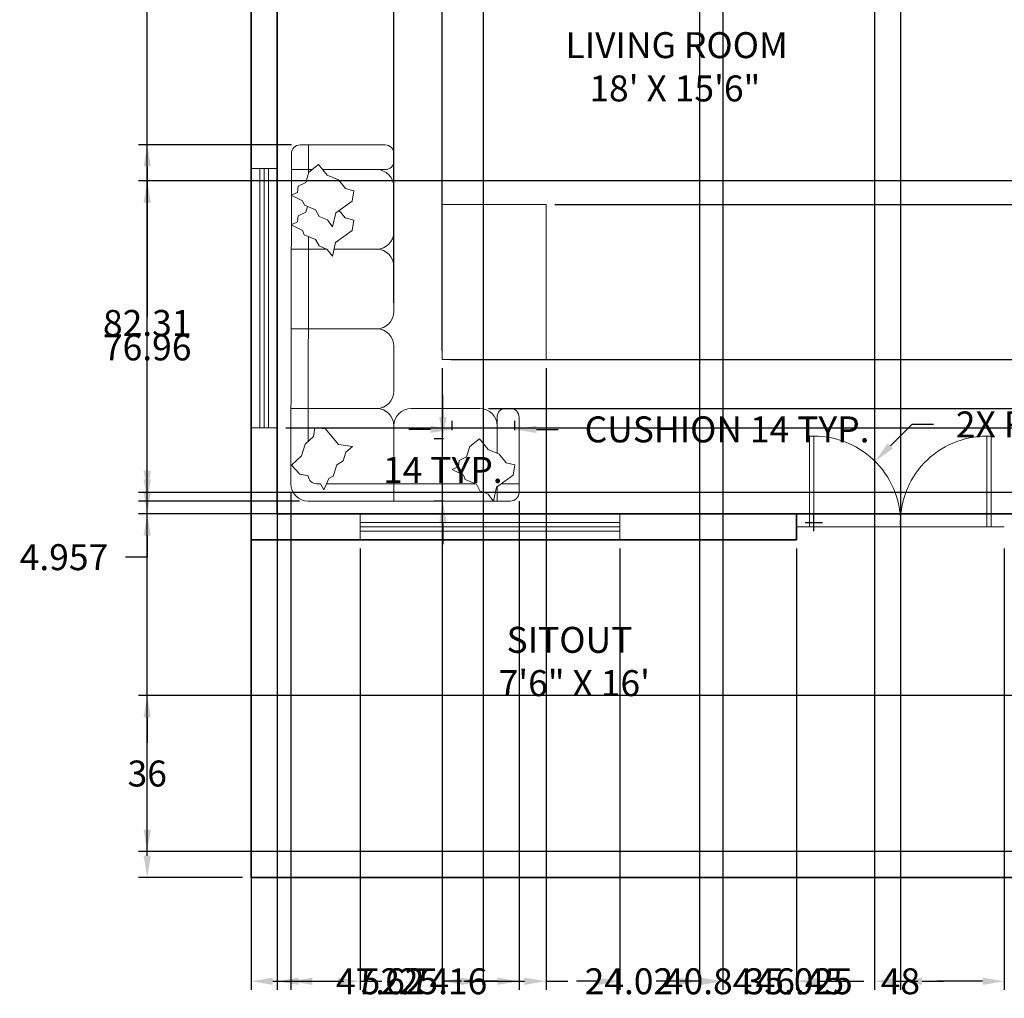
# Model space of a CAD drawing. Units: inches. Extents: x 185 to 668, y 153 to 689.
# Tile 1 of 5: x 190 to 417, y 153 to 380. Entities that reach past the tile are written whole.
import ezdxf

# ---------------------------------------------------------------- set-up
doc = ezdxf.new("R2010")
doc.units = ezdxf.units.IN
doc.header["$MEASUREMENT"] = 0
for name, color, linetype, lineweight in [('A-ANNO-DIMS', 2, 'Continuous', 18), ('A-AREA-IDEN', 7, 'Continuous', 25), ('A-DOOR', 3, 'Continuous', 18), ('A-FURN', 8, 'Continuous', 18), ('A-GLAZ', 4, 'Continuous', 18), ('A-WALL', 7, 'Continuous', 35)]:
    doc.layers.add(name, color=color, linetype=linetype, lineweight=lineweight)
doc.styles.get("Standard").update_dxf_attribs({"font": 'arial.ttf'})
doc.dimstyles.get("Standard").update_dxf_attribs({"dimtxt": 6, "dimasz": 5, "dimexe": 2, "dimexo": 2, "dimgap": 4, "dimtad": 0, "dimtih": 1, "dimtoh": 1, "dimdec": 0, "dimzin": 0, "dimdsep": 46, "dimlunit": 3, "dimtxsty": 'Standard', "dimcen": 2, "dimadec": 0, "dimazin": 0, "dimtfac": 1, "dimtdec": 0, "dimtofl": 0, "dimtmove": 0, "dimatfit": 3, "dimfxl": 1, "dimtolj": 1, "dimtzin": 0, "dimarcsym": 0})

# ---------------------------------------------------------------- blocks, each defined once
blk = doc.blocks.new('CUSHION-SOFA')
for p, q in [((6.28, 14.39), (4.07, 12.61)), ((6.28, 14.39), (8.27, 11.92)), ((4.07, 12.61), (3.33, 10.2)), ((8.27, 11.92), (10.87, 10.84)), ((1.59, 9.37), (1.41, 7.95)), ((3.33, 10.2), (1.59, 9.37)), ((10.87, 10.84), (12.49, 8.85)), ((1.41, 7.95), (0, 7.29)), ((0, 7.29), (2.58, 5.99)), ((12.49, 8.85), (14.45, 8.34)), ((14.09, 5.96), (14.45, 8.34)), ((2.58, 5.99), (3.01, 4.98)), ((3.01, 4.98), (5.57, 3.91)), ((10.25, 3.2), (14.09, 5.96)), ((5.57, 3.91), (6.41, 2.39)), ((6.41, 2.39), (8.33, 1.6)), ((9.53, 0), (10.25, 3.2)), ((8.33, 1.6), (9.53, 0))]:
    blk.add_line(p, q)
blk = doc.blocks.new('WINDOW-60')
for p, q in [((2, 60), (0, 60)), ((2, 60), (2, 0)), ((4, 60), (2, 60)), ((3, 0), (3, 60)), ((4, 0), (4, 60)), ((4, 60), (6, 60)), ((6, 0), (0, 0)), ((2, 0), (0, 0)), ((2, 0), (4, 0)), ((4, 0), (6, 0))]:
    blk.add_line(p, q)
blk = doc.blocks.new('*D17')
at = {"layer": 'A-ANNO-DIMS', "color": 0, "lineweight": -2, "transparency": 16777216}
for p, q in [((289.49, 284.74), (289.49, 286.91)), ((303.94, 284.74), (303.94, 286.91)), ((284.49, 284.91), (279.49, 284.91)), ((308.94, 284.91), (313.94, 284.91))]:
    blk.add_line(p, q, dxfattribs=at)
at = {"layer": 'A-ANNO-DIMS', "color": 0, "transparency": 16777216}
for points in [[(284.49, 285.74), (284.49, 284.08), (289.49, 284.91)], [(308.94, 285.74), (308.94, 284.08), (303.94, 284.91)]]:
    blk.add_solid(points, dxfattribs=at)
at = {"layer": 'Defpoints', "color": 0, "transparency": 16777216}
for p in [(303.94, 284.91), (289.49, 282.74), (303.94, 282.74)]:
    blk.add_point(p, dxfattribs=at)
at = {"layer": 'A-ANNO-DIMS', "color": 0, "transparency": 16777216, "insert": (352.99, 284.91), "char_height": 6, "attachment_point": 5}
blk.add_mtext('\\A1;CUSHION 14 TYP.', dxfattribs=at)
blk = doc.blocks.new('*D18')
at = {"layer": 'A-ANNO-DIMS', "color": 0, "lineweight": -2, "transparency": 16777216}
for p, q in [((287.32, 287.74), (287.32, 292.74)), ((287.49, 282.74), (285.32, 282.74)), ((287.49, 268.35), (285.32, 268.35)), ((287.32, 263.35), (287.32, 258.35))]:
    blk.add_line(p, q, dxfattribs=at)
at = {"layer": 'A-ANNO-DIMS', "color": 0, "transparency": 16777216}
for points in [[(286.49, 287.74), (288.16, 287.74), (287.32, 282.74)], [(286.49, 263.35), (288.16, 263.35), (287.32, 268.35)]]:
    blk.add_solid(points, dxfattribs=at)
at = {"layer": 'Defpoints', "color": 0, "transparency": 16777216}
for p in [(287.32, 282.74), (289.49, 282.74), (289.49, 268.35)]:
    blk.add_point(p, dxfattribs=at)
at = {"layer": 'A-ANNO-DIMS', "color": 0, "transparency": 16777216, "insert": (287.32, 275.55), "char_height": 6, "attachment_point": 5}
blk.add_mtext('\\A1;14 TYP.', dxfattribs=at)
blk = doc.blocks.new('*D26')
at = {"layer": 'A-ANNO-DIMS', "color": 0, "lineweight": -2, "transparency": 16777216}
for p, q in [((241.04, 661.38), (217.02, 661.38)), ((219.02, 656.38), (219.02, 428.44)), ((219.02, 186.38), (219.02, 414.32)), ((241.04, 181.38), (217.02, 181.38))]:
    blk.add_line(p, q, dxfattribs=at)
at = {"layer": 'A-ANNO-DIMS', "color": 0, "transparency": 16777216}
for points in [[(218.19, 656.38), (219.86, 656.38), (219.02, 661.38)], [(218.19, 186.38), (219.86, 186.38), (219.02, 181.38)]]:
    blk.add_solid(points, dxfattribs=at)
at = {"layer": 'Defpoints', "color": 0, "transparency": 16777216}
for p in [(219.02, 661.38), (243.04, 661.38), (243.04, 181.38)]:
    blk.add_point(p, dxfattribs=at)
at = {"layer": 'A-ANNO-DIMS', "color": 0, "transparency": 16777216, "insert": (219.02, 421.38), "char_height": 6, "attachment_point": 5}
blk.add_mtext('\\A1;480', dxfattribs=at)
blk = doc.blocks.new('*D28')
at = {"layer": 'A-ANNO-DIMS', "color": 0, "lineweight": -2, "transparency": 16777216}
for p, q in [((627.06, 285.24), (627.06, 290.24)), ((627.06, 290.24), (632.06, 290.24)), ((251.04, 285.24), (629.06, 285.24)), ((627.06, 270.38), (627.06, 280.24)), ((251.04, 265.38), (629.06, 265.38))]:
    blk.add_line(p, q, dxfattribs=at)
at = {"layer": 'A-ANNO-DIMS', "color": 0, "transparency": 16777216}
for points in [[(626.23, 280.24), (627.89, 280.24), (627.06, 285.24)], [(626.23, 270.38), (627.89, 270.38), (627.06, 265.38)]]:
    blk.add_solid(points, dxfattribs=at)
at = {"layer": 'Defpoints', "color": 0, "transparency": 16777216}
for p in [(249.04, 285.24), (627.06, 285.24), (249.04, 265.38)]:
    blk.add_point(p, dxfattribs=at)
at = {"layer": 'A-ANNO-DIMS', "color": 0, "transparency": 16777216, "insert": (645.9, 290.24), "char_height": 6, "attachment_point": 5}
blk.add_mtext('\\A1;19.86', dxfattribs=at)
blk = doc.blocks.new('*D32')
at = {"layer": 'A-ANNO-DIMS', "color": 0, "lineweight": -2, "transparency": 16777216}
for p, q in [((352.02, 653.38), (352.02, 155.36)), ((387.04, 653.38), (387.04, 155.36)), ((347.02, 157.36), (342.02, 157.36)), ((392.04, 157.36), (397.04, 157.36))]:
    blk.add_line(p, q, dxfattribs=at)
at = {"layer": 'A-ANNO-DIMS', "color": 0, "transparency": 16777216}
for points in [[(347.02, 158.19), (347.02, 156.53), (352.02, 157.36)], [(392.04, 158.19), (392.04, 156.53), (387.04, 157.36)]]:
    blk.add_solid(points, dxfattribs=at)
at = {"layer": 'Defpoints', "color": 0, "transparency": 16777216}
for p in [(352.02, 655.38), (387.04, 655.38), (387.04, 157.36)]:
    blk.add_point(p, dxfattribs=at)
at = {"layer": 'A-ANNO-DIMS', "color": 0, "transparency": 16777216, "insert": (369.53, 157.36), "char_height": 6, "attachment_point": 5}
blk.add_mtext('\\A1;35.025', dxfattribs=at)
blk = doc.blocks.new('*D34')
at = {"layer": 'A-ANNO-DIMS', "color": 0, "lineweight": -2, "transparency": 16777216}
for p, q in [((243.04, 257.38), (243.04, 155.36)), ((268.2, 257.38), (268.2, 155.36)), ((248.04, 157.36), (263.2, 157.36)), ((268.2, 157.36), (273.2, 157.36))]:
    blk.add_line(p, q, dxfattribs=at)
at = {"layer": 'A-ANNO-DIMS', "color": 0, "transparency": 16777216}
for points in [[(248.04, 158.19), (248.04, 156.53), (243.04, 157.36)], [(263.2, 158.19), (263.2, 156.53), (268.2, 157.36)]]:
    blk.add_solid(points, dxfattribs=at)
at = {"layer": 'Defpoints', "color": 0, "transparency": 16777216}
for p in [(243.04, 259.38), (268.2, 259.38), (268.2, 157.36)]:
    blk.add_point(p, dxfattribs=at)
at = {"layer": 'A-ANNO-DIMS', "color": 0, "transparency": 16777216, "insert": (287.37, 157.36), "char_height": 6, "attachment_point": 5}
blk.add_mtext('\\A1;25.16', dxfattribs=at)
blk = doc.blocks.new('*D35')
at = {"layer": 'A-ANNO-DIMS', "color": 0, "lineweight": -2, "transparency": 16777216}
for p, q in [((328.2, 257.38), (328.2, 155.36)), ((369.04, 257.38), (369.04, 155.36)), ((323.2, 157.36), (318.2, 157.36)), ((374.04, 157.36), (379.04, 157.36))]:
    blk.add_line(p, q, dxfattribs=at)
at = {"layer": 'A-ANNO-DIMS', "color": 0, "transparency": 16777216}
for points in [[(323.2, 158.19), (323.2, 156.53), (328.2, 157.36)], [(374.04, 158.19), (374.04, 156.53), (369.04, 157.36)]]:
    blk.add_solid(points, dxfattribs=at)
at = {"layer": 'Defpoints', "color": 0, "transparency": 16777216}
for p in [(328.2, 259.38), (369.04, 259.38), (369.04, 157.36)]:
    blk.add_point(p, dxfattribs=at)
at = {"layer": 'A-ANNO-DIMS', "color": 0, "transparency": 16777216, "insert": (348.62, 157.36), "char_height": 6, "attachment_point": 5}
blk.add_mtext('\\A1;40.84', dxfattribs=at)
blk = doc.blocks.new('*D36')
at = {"layer": 'A-ANNO-DIMS', "color": 0, "lineweight": -2, "transparency": 16777216}
for p, q in [((369.04, 257.38), (369.04, 155.36)), ((417.04, 257.38), (417.04, 155.36)), ((374.04, 157.36), (384.62, 157.36)), ((412.04, 157.36), (401.47, 157.36))]:
    blk.add_line(p, q, dxfattribs=at)
at = {"layer": 'A-ANNO-DIMS', "color": 0, "transparency": 16777216}
for points in [[(374.04, 158.19), (374.04, 156.53), (369.04, 157.36)], [(412.04, 158.19), (412.04, 156.53), (417.04, 157.36)]]:
    blk.add_solid(points, dxfattribs=at)
at = {"layer": 'Defpoints', "color": 0, "transparency": 16777216}
for p in [(369.04, 259.38), (417.04, 259.38), (417.04, 157.36)]:
    blk.add_point(p, dxfattribs=at)
at = {"layer": 'A-ANNO-DIMS', "color": 0, "transparency": 16777216, "insert": (393.04, 157.36), "char_height": 6, "attachment_point": 5}
blk.add_mtext('\\A1;48', dxfattribs=at)
blk = doc.blocks.new('*D53')
at = {"layer": 'A-ANNO-DIMS', "color": 0, "lineweight": -2, "transparency": 16777216}
for p, q in [((457.04, 342.34), (217.02, 342.34)), ((219.02, 337.34), (219.02, 310.92)), ((219.02, 270.38), (219.02, 296.79)), ((457.04, 265.38), (217.02, 265.38))]:
    blk.add_line(p, q, dxfattribs=at)
at = {"layer": 'A-ANNO-DIMS', "color": 0, "transparency": 16777216}
for points in [[(218.19, 337.34), (219.86, 337.34), (219.02, 342.34)], [(218.19, 270.38), (219.86, 270.38), (219.02, 265.38)]]:
    blk.add_solid(points, dxfattribs=at)
at = {"layer": 'Defpoints', "color": 0, "transparency": 16777216}
for p in [(219.02, 342.34), (459.04, 342.34), (459.04, 265.38)]:
    blk.add_point(p, dxfattribs=at)
at = {"layer": 'A-ANNO-DIMS', "color": 0, "transparency": 16777216, "insert": (219.02, 303.86), "char_height": 6, "attachment_point": 5}
blk.add_mtext('\\A1;76.96', dxfattribs=at)
blk = doc.blocks.new('*D54')
at = {"layer": 'A-ANNO-DIMS', "color": 0, "lineweight": -2, "transparency": 16777216}
for p, q in [((287.14, 299.05), (287.14, 155.36)), ((311.16, 299.05), (311.16, 155.36)), ((292.14, 157.36), (306.16, 157.36)), ((311.16, 157.36), (316.16, 157.36))]:
    blk.add_line(p, q, dxfattribs=at)
at = {"layer": 'A-ANNO-DIMS', "color": 0, "transparency": 16777216}
for points in [[(292.14, 158.19), (292.14, 156.53), (287.14, 157.36)], [(306.16, 158.19), (306.16, 156.53), (311.16, 157.36)]]:
    blk.add_solid(points, dxfattribs=at)
at = {"layer": 'Defpoints', "color": 0, "transparency": 16777216}
for p in [(287.14, 301.05), (311.16, 301.05), (311.16, 157.36)]:
    blk.add_point(p, dxfattribs=at)
at = {"layer": 'A-ANNO-DIMS', "color": 0, "transparency": 16777216, "insert": (330.3, 157.36), "char_height": 6, "attachment_point": 5}
blk.add_mtext('\\A1;24.02', dxfattribs=at)
blk = doc.blocks.new('*D55')
at = {"layer": 'A-ANNO-DIMS', "color": 0, "lineweight": -2, "transparency": 16777216}
for p, q in [((313.16, 336.85), (629.06, 336.85)), ((627.06, 331.85), (627.06, 326.02)), ((627.06, 306.05), (627.06, 311.89)), ((313.16, 301.05), (629.06, 301.05))]:
    blk.add_line(p, q, dxfattribs=at)
at = {"layer": 'A-ANNO-DIMS', "color": 0, "transparency": 16777216}
for points in [[(626.23, 331.85), (627.89, 331.85), (627.06, 336.85)], [(626.23, 306.05), (627.89, 306.05), (627.06, 301.05)]]:
    blk.add_solid(points, dxfattribs=at)
at = {"layer": 'Defpoints', "color": 0, "transparency": 16777216}
for p in [(311.16, 336.85), (627.06, 336.85), (311.16, 301.05)]:
    blk.add_point(p, dxfattribs=at)
at = {"layer": 'A-ANNO-DIMS', "color": 0, "transparency": 16777216, "insert": (627.06, 318.95), "char_height": 6, "attachment_point": 5}
blk.add_mtext('\\A1;35.8', dxfattribs=at)
blk = doc.blocks.new('*D56')
at = {"layer": 'A-ANNO-DIMS', "color": 0, "lineweight": -2, "transparency": 16777216}
for p, q in [((252.19, 270.35), (252.19, 155.36)), ((304.93, 268.35), (304.93, 155.36)), ((257.19, 157.36), (264.45, 157.36)), ((299.93, 157.36), (292.67, 157.36))]:
    blk.add_line(p, q, dxfattribs=at)
at = {"layer": 'A-ANNO-DIMS', "color": 0, "transparency": 16777216}
for points in [[(257.19, 158.19), (257.19, 156.53), (252.19, 157.36)], [(299.93, 158.19), (299.93, 156.53), (304.93, 157.36)]]:
    blk.add_solid(points, dxfattribs=at)
at = {"layer": 'Defpoints', "color": 0, "transparency": 16777216}
for p in [(252.19, 272.35), (304.93, 270.35), (304.93, 157.36)]:
    blk.add_point(p, dxfattribs=at)
at = {"layer": 'A-ANNO-DIMS', "color": 0, "transparency": 16777216, "insert": (278.56, 157.36), "char_height": 6, "attachment_point": 5}
blk.add_mtext('\\A1;52.74', dxfattribs=at)
blk = doc.blocks.new('*D57')
at = {"layer": 'A-ANNO-DIMS', "color": 0, "lineweight": -2, "transparency": 16777216}
for p, q in [((252.32, 350.67), (217.02, 350.67)), ((219.02, 345.67), (219.02, 316.58)), ((219.02, 273.35), (219.02, 302.45)), ((254.19, 268.35), (217.02, 268.35))]:
    blk.add_line(p, q, dxfattribs=at)
at = {"layer": 'A-ANNO-DIMS', "color": 0, "transparency": 16777216}
for points in [[(218.19, 345.67), (219.86, 345.67), (219.02, 350.67)], [(218.19, 273.35), (219.86, 273.35), (219.02, 268.35)]]:
    blk.add_solid(points, dxfattribs=at)
at = {"layer": 'Defpoints', "color": 0, "transparency": 16777216}
for p in [(219.02, 350.67), (254.32, 350.67), (256.19, 268.35)]:
    blk.add_point(p, dxfattribs=at)
at = {"layer": 'A-ANNO-DIMS', "color": 0, "transparency": 16777216, "insert": (219.02, 309.51), "char_height": 6, "attachment_point": 5}
blk.add_mtext('\\A1;82.31', dxfattribs=at)
blk = doc.blocks.new('*D58')
at = {"layer": 'A-ANNO-DIMS', "color": 0, "lineweight": -2, "transparency": 16777216}
for p, q in [((276.02, 314.15), (276.02, 687.4)), ((287.14, 303.05), (287.14, 687.4)), ((271.02, 685.4), (266.02, 685.4)), ((292.14, 685.4), (297.14, 685.4))]:
    blk.add_line(p, q, dxfattribs=at)
at = {"layer": 'A-ANNO-DIMS', "color": 0, "transparency": 16777216}
for points in [[(271.02, 686.23), (271.02, 684.56), (276.02, 685.4)], [(292.14, 686.23), (292.14, 684.56), (287.14, 685.4)]]:
    blk.add_solid(points, dxfattribs=at)
at = {"layer": 'Defpoints', "color": 0, "transparency": 16777216}
for p in [(287.14, 685.4), (276.02, 312.15), (287.14, 301.05)]:
    blk.add_point(p, dxfattribs=at)
at = {"layer": 'A-ANNO-DIMS', "color": 0, "transparency": 16777216, "insert": (313.31, 685.4), "char_height": 6, "attachment_point": 5}
blk.add_mtext('\\A1;11.116', dxfattribs=at)
blk = doc.blocks.new('*D59')
at = {"layer": 'A-ANNO-DIMS', "color": 0, "lineweight": -2, "transparency": 16777216}
for p, q in [((627.06, 306.05), (627.06, 311.05)), ((289.14, 301.05), (629.06, 301.05)), ((297.85, 289.75), (629.06, 289.75)), ((627.06, 284.75), (627.06, 279.75)), ((627.06, 279.75), (622.06, 279.75))]:
    blk.add_line(p, q, dxfattribs=at)
at = {"layer": 'A-ANNO-DIMS', "color": 0, "transparency": 16777216}
for points in [[(626.23, 306.05), (627.89, 306.05), (627.06, 301.05)], [(626.23, 284.75), (627.89, 284.75), (627.06, 289.75)]]:
    blk.add_solid(points, dxfattribs=at)
at = {"layer": 'Defpoints', "color": 0, "transparency": 16777216}
for p in [(287.14, 301.05), (295.85, 289.75), (627.06, 289.75)]:
    blk.add_point(p, dxfattribs=at)
at = {"layer": 'A-ANNO-DIMS', "color": 0, "transparency": 16777216, "insert": (605.89, 279.75), "char_height": 6, "attachment_point": 5}
blk.add_mtext('\\A1;11.303', dxfattribs=at)
blk = doc.blocks.new('*D60')
at = {"layer": 'A-ANNO-DIMS', "color": 0, "lineweight": -2, "transparency": 16777216}
for p, q in [((439.04, 223.38), (217.02, 223.38)), ((219.02, 218.38), (219.02, 212.44)), ((219.02, 192.38), (219.02, 198.31)), ((439.04, 187.38), (217.02, 187.38))]:
    blk.add_line(p, q, dxfattribs=at)
at = {"layer": 'A-ANNO-DIMS', "color": 0, "transparency": 16777216}
for points in [[(218.19, 218.38), (219.86, 218.38), (219.02, 223.38)], [(218.19, 192.38), (219.86, 192.38), (219.02, 187.38)]]:
    blk.add_solid(points, dxfattribs=at)
at = {"layer": 'Defpoints', "color": 0, "transparency": 16777216}
for p in [(219.02, 223.38), (441.04, 223.38), (441.04, 187.38)]:
    blk.add_point(p, dxfattribs=at)
at = {"layer": 'A-ANNO-DIMS', "color": 0, "transparency": 16777216, "insert": (219.02, 205.38), "char_height": 6, "attachment_point": 5}
blk.add_mtext('\\A1;36', dxfattribs=at)
blk = doc.blocks.new('*D70')
at = {"layer": 'A-ANNO-DIMS', "color": 0, "lineweight": -2, "transparency": 16777216}
for p, q in [((393.04, 479.38), (393.04, 155.36)), ((346.59, 452.48), (346.59, 155.36)), ((341.59, 157.36), (336.59, 157.36)), ((398.04, 157.36), (403.04, 157.36))]:
    blk.add_line(p, q, dxfattribs=at)
at = {"layer": 'A-ANNO-DIMS', "color": 0, "transparency": 16777216}
for points in [[(341.59, 158.19), (341.59, 156.53), (346.59, 157.36)], [(398.04, 158.19), (398.04, 156.53), (393.04, 157.36)]]:
    blk.add_solid(points, dxfattribs=at)
at = {"layer": 'Defpoints', "color": 0, "transparency": 16777216}
for p in [(393.04, 481.38), (346.59, 454.48), (393.04, 157.36)]:
    blk.add_point(p, dxfattribs=at)
at = {"layer": 'A-ANNO-DIMS', "color": 0, "transparency": 16777216, "insert": (369.81, 157.36), "char_height": 6, "attachment_point": 5}
blk.add_mtext('\\A1;46.45', dxfattribs=at)
blk = doc.blocks.new('*D72')
at = {"layer": 'A-ANNO-DIMS', "color": 0, "lineweight": -2, "transparency": 16777216}
for p, q in [((249.04, 653.38), (249.04, 155.36)), ((296.66, 647.15), (296.66, 155.36)), ((254.04, 157.36), (258.64, 157.36)), ((291.66, 157.36), (287.06, 157.36))]:
    blk.add_line(p, q, dxfattribs=at)
at = {"layer": 'A-ANNO-DIMS', "color": 0, "transparency": 16777216}
for points in [[(254.04, 158.19), (254.04, 156.53), (249.04, 157.36)], [(291.66, 158.19), (291.66, 156.53), (296.66, 157.36)]]:
    blk.add_solid(points, dxfattribs=at)
at = {"layer": 'Defpoints', "color": 0, "transparency": 16777216}
for p in [(249.04, 655.38), (296.66, 649.15), (296.66, 157.36)]:
    blk.add_point(p, dxfattribs=at)
at = {"layer": 'A-ANNO-DIMS', "color": 0, "transparency": 16777216, "insert": (272.85, 157.36), "char_height": 6, "attachment_point": 5}
blk.add_mtext('\\A1;47.62', dxfattribs=at)
blk = doc.blocks.new('*D75')
at = {"layer": 'A-ANNO-DIMS', "color": 0, "lineweight": -2, "transparency": 16777216}
for p, q in [((219.02, 275.34), (219.02, 280.34)), ((559.08, 270.34), (217.02, 270.34)), ((595.04, 265.38), (217.02, 265.38)), ((219.02, 260.38), (219.02, 255.38)), ((219.02, 255.38), (214.02, 255.38))]:
    blk.add_line(p, q, dxfattribs=at)
at = {"layer": 'A-ANNO-DIMS', "color": 0, "transparency": 16777216}
for points in [[(218.19, 275.34), (219.86, 275.34), (219.02, 270.34)], [(218.19, 260.38), (219.86, 260.38), (219.02, 265.38)]]:
    blk.add_solid(points, dxfattribs=at)
at = {"layer": 'Defpoints', "color": 0, "transparency": 16777216}
for p in [(561.08, 270.34), (219.02, 265.38), (597.04, 265.38)]:
    blk.add_point(p, dxfattribs=at)
at = {"layer": 'A-ANNO-DIMS', "color": 0, "transparency": 16777216, "insert": (199.78, 255.38), "char_height": 6, "attachment_point": 5}
blk.add_mtext('\\A1;4.957', dxfattribs=at)
blk = doc.blocks.new('*D76')
at = {"layer": 'A-ANNO-DIMS', "color": 0, "lineweight": -2, "transparency": 16777216}
for p, q in [((395.66, 286.05), (390.71, 281.08)), ((400.66, 286.05), (395.66, 286.05)), ((373.04, 261.36), (373.04, 265.36)), ((371.04, 263.36), (375.04, 263.36))]:
    blk.add_line(p, q, dxfattribs=at)
at = {"layer": 'A-ANNO-DIMS', "color": 0, "transparency": 16777216}
blk.add_solid([(390.12, 281.67), (391.3, 280.49), (387.18, 277.54)], dxfattribs=at)
at = {"layer": 'Defpoints', "color": 0, "transparency": 16777216}
for p in [(387.18, 277.54), (373.04, 263.36)]:
    blk.add_point(p, dxfattribs=at)
at = {"layer": 'A-ANNO-DIMS', "color": 0, "transparency": 16777216, "insert": (426.47, 286.05), "char_height": 6, "attachment_point": 5}
blk.add_mtext('\\A1;2X R20.024', dxfattribs=at)

msp = doc.modelspace()

# ---------------------------------------------------------------- linework, layer by layer
at = {"layer": 'A-DOOR'}
for p, q in [((372.041, 262.3789), (372.041, 283.3789)), ((372.041, 283.3789), (373.041, 283.3789)), ((373.041, 283.3789), (373.041, 262.3789)), ((414.041, 283.3789), (413.041, 283.3789)), ((413.041, 283.3789), (413.041, 262.3789)), ((414.041, 262.3789), (414.041, 283.3789)), ((369.041, 262.3789), (372.041, 262.3789)), ((372.041, 262.3789), (414.041, 262.3789)), ((417.041, 262.3789), (414.041, 262.3789))]:
    msp.add_line(p, q, dxfattribs=at)
for centre, start, end in [((373.041, 263.3551), 357.205638, 90), ((413.041, 263.3551), 90, 182.794362)]:
    msp.add_arc(centre, 20.0238, start, end, dxfattribs=at)
at = {"layer": 'A-FURN'}
for p, q in [((254.324, 350.6678), (274.02, 350.6678)), ((256.2937, 344.9426), (256.2937, 350.6678)), ((252.324, 345.595), (252.324, 348.6678)), ((276.02, 348.6678), (276.02, 346.9426)), ((252.324, 345.595), (252.186, 272.3537)), ((252.3228, 344.9426), (257.1256, 344.9426)), ((252.324, 345.595), (252.324, 345.595)), ((256.2937, 344.0609), (256.2937, 344.9426)), ((259.5443, 344.9426), (272.02, 344.9426)), ((272.02, 344.9426), (274.02, 344.9426)), ((276.02, 340.9426), (276.02, 330.5454)), ((255.6303, 335.1219), (253.8892, 334.2881)), ((256.0282, 336.422), (255.6303, 335.1219)), ((263.3703, 335.5123), (264.785, 333.7672)), ((253.7057, 332.8677), (252.2988, 332.2079)), ((252.2988, 332.2079), (254.8782, 330.914)), ((253.8892, 334.2881), (253.7057, 332.8677)), ((264.785, 333.7672), (266.7454, 333.2637)), ((266.386, 330.8762), (266.7454, 333.2637)), ((254.8782, 330.914), (255.313, 329.9034)), ((255.313, 329.9034), (257.8645, 328.8322)), ((262.551, 328.119), (266.386, 330.8762)), ((256.2937, 329.4917), (256.2044, 282.13)), ((257.8645, 328.8322), (258.7101, 327.3063)), ((261.8319, 324.9195), (262.551, 328.119)), ((252.2881, 326.5454), (260.5643, 326.5454)), ((260.5643, 326.5454), (252.2881, 326.5454)), ((258.7101, 327.3063), (260.6247, 326.5206)), ((260.6247, 326.5206), (261.8319, 324.9195)), ((272.02, 326.5454), (262.1973, 326.5454)), ((262.1973, 326.5454), (272.02, 326.5454)), ((276.02, 322.5454), (276.02, 312.1481)), ((272.02, 308.1481), (252.2535, 308.1481)), ((252.2535, 308.1481), (272.02, 308.1481)), ((276.02, 304.1481), (276.02, 293.7509)), ((252.2188, 289.7509), (272.02, 289.7509)), ((272.02, 289.7509), (252.2188, 289.7509)), ((280.02, 289.7509), (295.8541, 289.7509)), ((302.9269, 289.7561), (301.8541, 289.7561)), ((299.8541, 287.7561), (299.8541, 279.407)), ((304.9269, 270.3537), (304.9269, 287.7561)), ((257.4036, 283.2553), (257.7641, 285.247)), ((260.1713, 285.0612), (257.7641, 285.247)), ((263.1986, 281.4357), (260.1713, 285.0612)), ((276.02, 285.7509), (276.02, 268.3537)), ((276.02, 268.3537), (276.02, 285.7509)), ((299.8541, 285.7509), (299.8541, 279.407)), ((255.5288, 281.496), (257.4036, 283.2553)), ((254.641, 278.8251), (255.5288, 281.496)), ((266.4418, 280.9498), (263.1986, 281.4357)), ((264.9322, 279.63), (266.4418, 280.9498)), ((252.3237, 276.6667), (254.641, 278.8251)), ((262.8262, 276.7098), (264.287, 277.6635)), ((264.287, 277.6635), (264.9322, 279.63)), ((252.3237, 276.6667), (254.2604, 274.5873)), ((261.9423, 274.0875), (262.8262, 276.7098)), ((254.2604, 274.5873), (256.2008, 274.144)), ((259.8619, 270.9146), (260.9659, 273.5808)), ((260.9659, 273.5808), (261.9423, 274.0875)), ((259.0481, 272.3537), (258.1898, 272.3537)), ((259.0481, 272.3537), (259.8619, 270.9146)), ((294.8471, 272.3537), (260.4578, 272.3537)), ((299.8541, 271.6341), (299.8541, 268.3537)), ((304.9269, 272.3537), (300.8549, 272.3537)), ((272.02, 268.3537), (256.186, 268.3537)), ((295.8541, 268.3537), (256.186, 268.3537)), ((295.8541, 268.3537), (302.9269, 268.3537))]:
    msp.add_line(p, q, dxfattribs=at)
msp.add_lwpolyline([(287.1365, 336.854), (311.1562, 336.854), (311.1562, 301.0535), (287.1365, 301.0535)], close=True, dxfattribs=at)
for centre, radius, start, end in [((254.324, 348.6678), 2, 90, 180), ((274.02, 348.6678), 2, 0, 90), ((274.02, 346.9426), 2, 270, 0), ((272.02, 340.9426), 4, 0, 90), ((272.02, 330.5454), 4, 270, 0), ((272.02, 322.5454), 4, 0, 90), ((272.02, 312.1481), 4, 270, 0), ((272.02, 304.1481), 4, 0, 90), ((272.02, 293.7509), 4, 270, 0), ((272.02, 285.7509), 4, 0, 90), ((280.02, 285.7509), 4, 90, 180), ((295.8541, 285.7509), 4, 0, 90), ((301.8541, 287.7561), 2, 90, 180), ((302.9269, 287.7561), 2, 0, 90), ((258.1898, 274.3537), 2, 186.018077, 270), ((256.186, 272.3537), 4, 180, 270), ((302.9269, 270.3537), 2, 270, 0)]:
    msp.add_arc(centre, radius, start, end, dxfattribs=at)
at = {"layer": 'A-WALL'}
for p, q in [((243.041, 661.3789), (243.041, 181.3789)), ((249.041, 481.3789), (249.041, 265.3789)), ((369.041, 265.3789), (249.041, 265.3789)), ((369.041, 265.3789), (369.041, 259.3789)), ((243.041, 259.3789), (243.041, 181.3789)), ((369.041, 259.3789), (243.041, 259.3789)), ((243.041, 181.3789), (603.041, 181.3789))]:
    msp.add_line(p, q, dxfattribs=at)

# ---------------------------------------------------------------- block references
at = {"layer": 'A-FURN'}
for p in [(252.312, 331.733), (289.4896, 268.3537)]:
    msp.add_blockref('CUSHION-SOFA', p, dxfattribs=at)
at = {"layer": 'A-GLAZ'}
msp.add_blockref('WINDOW-60', (243.041, 285.239), dxfattribs=at)
at = {"layer": 'A-GLAZ', "rotation": 269.9999999999999}
msp.add_blockref('WINDOW-60', (268.1999, 265.3789), dxfattribs=at)

# ---------------------------------------------------------------- texts
at = {"layer": 'A-AREA-IDEN', "char_height": 6, "attachment_point": 1}
for s, insert in [('LIVING ROOM\\P   18\' X 15\'6"', (315.6763, 376.7146)), (' SITOUT\\P7\'6" X 16\'', (300.2084, 239.2715))]:
    msp.add_mtext_dynamic_manual_height_columns(s, width=69.605686, gutter_width=1, heights=[0], dxfattribs=dict(at, insert=insert))

# ---------------------------------------------------------------- dimensions: what is measured, and where the dimension line sits
at = {"layer": 'A-ANNO-DIMS'}
for base, p1, p2, override, picture, middle in [((287.13651, 685.39645), (276.02002, 312.14814), (287.13651, 301.05349), {"dimdec": 3, "dimlfac": 1, "dimrnd": 0, "dimzin": 0, "dimdsep": 46, "dimlunit": 2}, '*D58', (313.30636, 685.39645)), ((296.6583, 157.3614), (249.041, 655.3789), (296.6583, 649.1496), {"dimdec": 2, "dimlfac": 1, "dimrnd": 0, "dimzin": 0, "dimdsep": 46, "dimlunit": 2}, '*D72', (272.8496, 157.3614)), ((387.041, 157.3614), (352.0164, 655.3789), (387.041, 655.3789), {"dimdec": 3, "dimlfac": 1, "dimrnd": 0, "dimzin": 0, "dimdsep": 46, "dimlunit": 2}, '*D32', (369.5287, 157.3614)), ((393.041, 157.3614), (346.5866, 454.4811), (393.041, 481.3789), {"dimdec": 2, "dimlfac": 1, "dimrnd": 0, "dimzin": 0, "dimdsep": 46, "dimlunit": 2}, '*D70', (369.8138, 157.3614)), ((311.1562, 157.3614), (287.1365, 301.0535), (311.1562, 301.0535), {"dimdec": 2, "dimlfac": 1, "dimrnd": 0, "dimzin": 0, "dimdsep": 46, "dimlunit": 2}, '*D54', (330.3002, 157.3614)), ((304.9269, 157.3614), (252.186, 272.3537), (304.9269, 270.3537), {"dimdec": 2, "dimlfac": 1, "dimrnd": 0, "dimzin": 0, "dimdsep": 46, "dimlunit": 2}, '*D56', (278.5564, 157.3614)), ((268.1997, 157.3614), (243.041, 259.3789), (268.1997, 259.3789), {"dimdec": 2, "dimlfac": 1, "dimrnd": 0, "dimzin": 0, "dimdsep": 46, "dimlunit": 2}, '*D34', (287.3723, 157.3614)), ((369.041, 157.3614), (328.1997, 259.3789), (369.041, 259.3789), {"dimdec": 2, "dimlfac": 1, "dimrnd": 0, "dimzin": 0, "dimdsep": 46, "dimlunit": 2}, '*D35', (348.6203, 157.3614)), ((417.041, 157.3614), (369.041, 259.3789), (417.041, 259.3789), {"dimdec": 0, "dimlfac": 1, "dimrnd": 0, "dimzin": 0, "dimdsep": 46, "dimlunit": 2}, '*D36', (393.041, 157.3614))]:
    dim = msp.add_linear_dim(base=base, p1=p1, p2=p2, dimstyle='Standard', override=override, dxfattribs=at)
    dim.commit()
    dim.dimension.update_dxf_attribs({"geometry": picture, "text_midpoint": middle})
for base, p1, p2, override, picture, middle in [((219.0235, 661.3789), (243.041, 181.3789), (243.041, 661.3789), {"dimdec": 0, "dimlfac": 1, "dimrnd": 0, "dimzin": 0, "dimdsep": 46, "dimlunit": 2}, '*D26', (219.0235, 421.3789)), ((219.0235, 350.6678), (256.186, 268.3537), (254.324, 350.6678), {"dimdec": 2, "dimlfac": 1, "dimrnd": 0, "dimzin": 0, "dimdsep": 46, "dimlunit": 2}, '*D57', (219.0235, 309.5108)), ((219.0235, 342.3357), (459.041, 265.3789), (459.041, 342.3357), {"dimdec": 2, "dimlfac": 1, "dimrnd": 0, "dimzin": 0, "dimdsep": 46, "dimlunit": 2}, '*D53', (219.0235, 303.8573)), ((627.0585, 336.854), (311.1562, 301.0535), (311.1562, 336.854), {"dimdec": 1, "dimlfac": 1, "dimrnd": 0, "dimzin": 0, "dimdsep": 46, "dimlunit": 2}, '*D55', (627.0585, 318.9537)), ((627.0585, 289.7509), (287.1365, 301.0535), (295.8541, 289.7509), {"dimdec": 3, "dimlfac": 1, "dimrnd": 0, "dimzin": 0, "dimdsep": 46, "dimlunit": 2}, '*D59', (605.8866, 279.7509)), ((627.0585, 285.2389), (249.041, 265.3789), (249.041, 285.2389), {"dimdec": 2, "dimlfac": 1, "dimrnd": 0, "dimzin": 0, "dimdsep": 46, "dimlunit": 2}, '*D28', (645.8975, 290.2389)), ((219.0235, 265.3789), (561.0793, 270.3357), (597.041, 265.3789), {"dimdec": 3, "dimlfac": 1, "dimrnd": 0, "dimzin": 0, "dimdsep": 46, "dimlunit": 2}, '*D75', (199.7793, 255.3789)), ((219.0235, 223.3789), (441.041, 187.3789), (441.041, 223.3789), {"dimdec": 0, "dimlfac": 1, "dimrnd": 0, "dimzin": 0, "dimdsep": 46, "dimlunit": 2}, '*D60', (219.0235, 205.3789))]:
    dim = msp.add_linear_dim(base=base, p1=p1, p2=p2, angle=90, dimstyle='Standard', override=override, dxfattribs=at)
    dim.commit()
    dim.dimension.update_dxf_attribs({"geometry": picture, "text_midpoint": middle})
dim = msp.add_linear_dim(base=(303.9358, 284.9115), p1=(289.4892, 282.7446), p2=(303.9358, 282.7446), text='CUSHION <> TYP.', dimstyle='Standard', override={"dimdec": 0, "dimlfac": 1, "dimrnd": 0, "dimzin": 0, "dimdsep": 46, "dimlunit": 2}, dxfattribs=at)
dim.commit()
dim.dimension.update_dxf_attribs({"geometry": '*D17', "text_midpoint": (352.9945, 284.9115)})
dim = msp.add_radius_dim(center=(373.041, 263.3551), mpoint=(387.1765, 277.5375), text='2X <>', dimstyle='Standard', override={"dimdec": 3, "dimlfac": 1, "dimrnd": 0, "dimzin": 0, "dimdsep": 46, "dimlunit": 2}, dxfattribs=at)
dim.commit()
dim.dimension.update_dxf_attribs({"geometry": '*D76', "text_midpoint": (426.4682, 286.0469), "dimtype": 164})
dim = msp.add_linear_dim(base=(287.3223, 282.7446), p1=(289.4892, 268.3537), p2=(289.4892, 282.7446), angle=90, text='<> TYP.', dimstyle='Standard', override={"dimdec": 0, "dimlfac": 1, "dimrnd": 0, "dimzin": 0, "dimdsep": 46, "dimlunit": 2}, dxfattribs=at)
dim.commit()
dim.dimension.update_dxf_attribs({"geometry": '*D18', "text_midpoint": (287.3223, 275.5491)})

doc.saveas('drawing.dxf')
